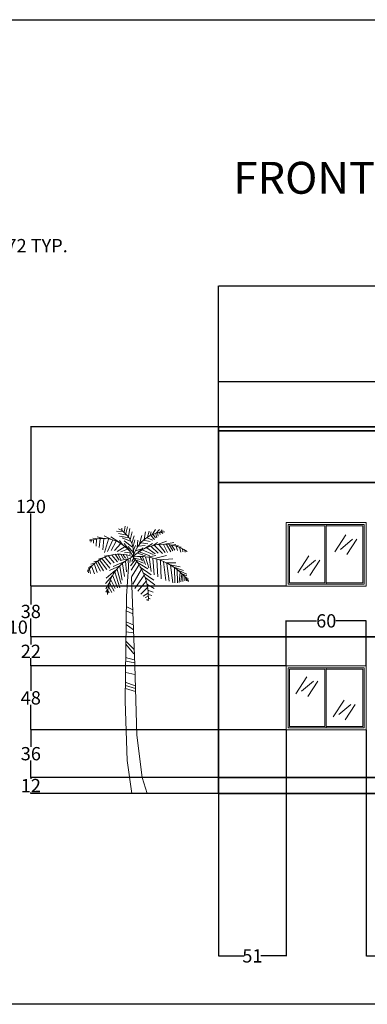
# Model space of a CAD drawing. Units: inches. Extents: x -16 to 1298, y 3 to 744.
# Tile 4 of 5: x 520 to 781, y 3 to 744. Entities that reach past the tile are written whole.
import ezdxf

# ---------------------------------------------------------------- set-up
doc = ezdxf.new("R2010")
doc.units = ezdxf.units.IN
doc.header["$MEASUREMENT"] = 0
for name, color, linetype, lineweight in [('A-ANNO-DIMS', 2, 'Continuous', 18), ('A-ANNO-TITL', 7, 'Continuous', 35), ('A-ELEV', 7, 'Continuous', 35), ('A-GLAZ', 4, 'Continuous', 18), ('A-ROOF', 7, 'Continuous', 35), ('C-TOPO', 7, 'Continuous', 30), ('PLANT', 3, 'Continuous', 13)]:
    doc.layers.add(name, color=color, linetype=linetype, lineweight=lineweight)
doc.styles.get("Standard").update_dxf_attribs({"font": 'arial.ttf'})
doc.dimstyles.get("Standard").update_dxf_attribs({"dimtxt": 10, "dimasz": 0.18, "dimexe": 0.18, "dimexo": 0.0625, "dimgap": 0.09, "dimtad": 0, "dimtih": 1, "dimtoh": 1, "dimdec": 0, "dimzin": 0, "dimdsep": 46, "dimlunit": 3, "dimtxsty": 'Standard', "dimcen": 0.09, "dimadec": 0, "dimazin": 0, "dimtfac": 1, "dimtdec": 0, "dimtofl": 0, "dimtmove": 0, "dimatfit": 3, "dimfxl": 1, "dimtolj": 1, "dimtzin": 0, "dimarcsym": 0})

# ---------------------------------------------------------------- blocks, each defined once
blk = doc.blocks.new('*U11')
for p, q in [((1.5, 1.5), (1.5, 46.5)), ((1.5, 46.5), (30, 46.5)), ((30, 1.5), (30, 46.5)), ((30, 46.5), (58.5, 46.5)), ((58.5, 46.5), (58.5, 1.5)), ((30, 1.5), (1.5, 1.5)), ((58.5, 1.5), (30, 1.5))]:
    blk.add_line(p, q)
blk.add_lwpolyline([(0, 0), (0, 48), (60, 48), (60, 0)], close=True)
for points in [[(29, 45.5), (29, 2.5), (2.5, 2.5), (2.5, 45.5), (29, 45.5)], [(30, 45.5), (57.5, 45.5), (57.5, 2.5), (30, 2.5)]]:
    blk.add_lwpolyline(points)
blk = doc.blocks.new('Tree - palm elevation')
for p, q in [((-5.567, 196.707), (-4.987, 201.167)), ((-4.407, 195.716), (-3.247, 200.672)), ((-20.064, 191.751), (-25.863, 193.238)), ((-15.232, 191.255), (-20.644, 193.981)), ((-9.433, 189.025), (-15.618, 193.238)), ((-6.727, 197.202), (-11.366, 197.45)), ((-3.441, 194.477), (-10.013, 195.716)), ((-1.894, 192.494), (-9.24, 193.733)), ((-7.5, 199.68), (-7.5, 197.946)), ((-2.474, 193.733), (-1.315, 199.433)), ((-1.121, 190.759), (0.232, 196.955)), ((0.038, 188.281), (1.778, 193.981)), ((5.837, 187.786), (7.577, 194.229)), ((9.317, 191.255), (10.283, 196.955)), ((11.829, 192.99), (13.182, 197.45)), ((13.956, 194.229), (14.729, 196.955)), ((14.536, 193.981), (17.242, 191.255)), ((15.116, 194.477), (17.822, 198.689)), ((16.082, 194.972), (17.822, 192.494)), ((18.015, 195.716), (20.914, 198.689)), ((18.015, 195.468), (18.981, 192.494)), ((19.368, 196.459), (19.948, 193.733)), ((20.914, 196.459), (21.301, 194.972)), ((21.301, 196.459), (22.847, 198.441)), ((22.074, 196.707), (23.427, 195.716)), ((23.234, 196.707), (23.62, 197.698)), ((-29.729, 190.759), (-31.469, 191.255)), ((-30.309, 190.512), (-30.695, 189.025)), ((-25.283, 191.751), (-29.342, 192.246)), ((-28.763, 190.759), (-28.763, 188.281)), ((-26.443, 191.503), (-26.636, 186.051)), ((-23.737, 191.751), (-24.51, 185.06)), ((-21.031, 191.998), (-21.804, 183.325)), ((-17.551, 191.503), (-20.451, 181.343)), ((-14.265, 190.759), (-18.131, 182.086)), ((-11.753, 189.768), (-15.425, 182.83)), ((-8.08, 188.034), (-12.912, 182.83)), ((-4.987, 185.803), (-10.979, 182.086)), ((-6.147, 186.299), (-9.24, 190.264)), ((-0.541, 189.52), (-7.307, 192.494)), ((-5.76, 190.016), (0.618, 185.308)), ((-5.76, 188.034), (-1.508, 182.582)), ((-2.668, 185.803), (1.198, 181.343)), ((1.005, 185.803), (2.358, 190.759)), ((1.005, 182.582), (2.938, 186.547)), ((4.098, 185.06), (4.678, 190.512)), ((4.871, 186.051), (10.09, 186.547)), ((6.997, 188.529), (12.216, 187.786)), ((8.544, 190.512), (13.763, 189.52)), ((9.51, 184.317), (15.502, 188.034)), ((11.25, 192.494), (15.889, 190.512)), ((14.536, 185.803), (19.948, 180.847)), ((15.695, 186.299), (19.368, 188.777)), ((17.242, 186.547), (23.041, 180.599)), ((19.368, 187.29), (26.133, 189.768)), ((20.721, 187.042), (25.167, 181.343)), ((23.814, 187.29), (26.907, 181.343)), ((24.78, 187.538), (31.546, 188.777)), ((26.133, 187.29), (29.419, 181.838)), ((28.066, 187.29), (30.966, 182.582)), ((29.806, 186.795), (32.319, 183.078)), ((29.999, 186.795), (33.092, 187.29)), ((32.512, 186.299), (35.218, 186.299)), ((33.479, 186.051), (34.445, 182.83)), ((35.605, 185.556), (37.151, 185.308)), ((35.798, 185.308), (36.958, 181.591)), ((-15.618, 179.36), (-20.644, 178.617)), ((-17.358, 178.617), (-13.299, 173.661)), ((-15.038, 179.36), (-10.786, 174.404)), ((-12.332, 180.104), (-9.433, 175.643)), ((-10.206, 180.104), (-8.08, 175.891)), ((-8.273, 180.104), (-6.147, 176.635)), ((-3.247, 183.821), (-8.08, 181.838)), ((-6.34, 179.608), (-4.6, 177.13)), ((-1.315, 181.591), (-5.374, 181.095)), ((-4.021, 179.36), (-2.861, 177.378)), ((-0.348, 180.352), (-1.894, 180.104)), ((2.938, 182.582), (6.61, 183.821)), ((4.098, 180.847), (8.35, 179.608)), ((4.871, 181.591), (8.544, 184.812)), ((5.644, 181.838), (13.569, 178.865)), ((6.224, 178.121), (8.157, 175.148)), ((7.384, 178.369), (10.476, 179.36)), ((7.77, 183.325), (16.082, 179.856)), ((8.157, 178.121), (10.476, 172.422)), ((10.476, 177.874), (12.796, 169.696)), ((11.25, 184.812), (17.628, 180.352)), ((11.829, 177.874), (18.015, 179.113)), ((13.182, 177.874), (14.729, 166.97)), ((18.015, 177.13), (26.133, 179.113)), ((38.118, 184.317), (38.504, 181.838)), ((39.857, 182.83), (40.244, 181.591)), ((-28.956, 172.174), (-32.435, 170.192)), ((-27.409, 173.413), (-30.695, 172.67)), ((-29.922, 170.687), (-27.989, 165.235)), ((-25.09, 175.148), (-28.376, 174.404)), ((-27.989, 172.422), (-26.056, 166.227)), ((-26.829, 173.661), (-23.544, 167.218)), ((-25.476, 174.652), (-21.224, 167.466)), ((-21.031, 177.626), (-24.897, 176.387)), ((-24.317, 175.891), (-18.711, 168.457)), ((-22.191, 176.635), (-16.391, 169.448)), ((-20.064, 177.626), (-15.812, 172.67)), ((-8.466, 171.678), (-16.585, 167.713)), ((-4.214, 175.148), (-14.072, 170.935)), ((-8.853, 170.935), (-7.113, 160.527)), ((-1.701, 176.882), (-8.66, 175.396)), ((-6.92, 172.917), (-5.374, 163.253)), ((-4.6, 174.9), (-4.021, 166.722)), ((-2.668, 176.387), (-2.376, 170.594)), ((-0.928, 176.882), (-1.508, 173.909)), ((2.551, 175.891), (-0.928, 171.431)), ((3.711, 174.404), (-0.541, 167.961)), ((5.257, 171.926), (-0.155, 163.005)), ((1.585, 177.13), (0.038, 174.652)), ((1.585, 177.13), (6.61, 176.139)), ((2.938, 175.891), (8.737, 173.413)), ((4.291, 173.909), (12.216, 168.953)), ((6.417, 170.439), (14.729, 164.492)), ((15.889, 177.13), (16.855, 164.492)), ((18.981, 175.891), (19.561, 163.005)), ((20.914, 175.891), (30.966, 176.635)), ((21.688, 175.396), (22.074, 161.518)), ((23.814, 174.404), (25.554, 160.279)), ((25.554, 173.661), (33.285, 173.661)), ((26.52, 173.165), (28.066, 159.784)), ((28.839, 172.174), (36.378, 170.687)), ((29.226, 171.926), (30.966, 158.545)), ((30.966, 170.687), (38.891, 167.713)), ((-32.628, 167.961), (-33.208, 167.961)), ((-32.628, 167.713), (-32.435, 165.979)), ((-31.082, 169.944), (-32.435, 169.2)), ((-31.662, 168.705), (-31.082, 165.483)), ((-14.265, 164.244), (-19.678, 158.049)), ((-12.139, 167.961), (-19.098, 162.014)), ((-14.265, 163.749), (-10.786, 154.828)), ((-12.719, 166.722), (-9.046, 154.828)), ((-10.979, 168.457), (-7.887, 157.801)), ((7.384, 168.705), (0.812, 157.553)), ((9.317, 164.244), (2.358, 154.332)), ((8.544, 165.979), (16.662, 160.527)), ((32.126, 169.696), (32.512, 158.545)), ((34.058, 168.705), (34.445, 158.545)), ((35.412, 167.713), (41.404, 164.988)), ((36.378, 166.474), (35.605, 158.792)), ((37.731, 165.235), (36.958, 159.288)), ((37.924, 165.235), (41.404, 163.749)), ((38.504, 164.492), (38.504, 159.536)), ((39.664, 163.253), (42.37, 161.766)), ((-16.005, 160.031), (-19.484, 154.084)), ((-17.358, 155.819), (-14.845, 151.358)), ((-16.585, 158.545), (-13.106, 152.35)), ((-15.618, 160.775), (-12.332, 154.332)), ((10.863, 159.784), (4.484, 152.35)), ((10.09, 162.51), (17.435, 157.058)), ((11.443, 157.553), (16.855, 154.332)), ((39.857, 162.757), (39.857, 160.031)), ((40.824, 161.766), (41.21, 160.031)), ((41.21, 161.518), (42.757, 160.279)), ((-18.131, 153.589), (-19.484, 151.606)), ((-17.938, 152.597), (-16.972, 151.111)), ((11.829, 155.075), (6.804, 150.119)), ((12.603, 151.111), (8.544, 148.385)), ((12.216, 153.093), (16.082, 151.606)), ((12.603, 149.872), (15.116, 149.128)), ((12.216, 148.137), (10.09, 147.393)), ((12.409, 145.659), (11.056, 145.659)), ((12.409, 146.898), (13.763, 146.402)), ((-4.081, 140.645), (0.753, 138.261)), ((-4.081, 137.547), (0.753, 135.163)), ((-4.081, 129.205), (1.124, 126.821)), ((-4.081, 127.298), (1.31, 123.246)), ((-4.081, 121.578), (1.31, 120.863)), ((-4.453, 112.283), (1.682, 105.133)), ((-4.267, 114.428), (1.682, 108.708)), ((-4.639, 102.273), (1.868, 100.604)), ((-4.453, 99.651), (2.24, 98.459)), ((-4.453, 91.071), (2.426, 89.641)), ((-4.825, 83.921), (2.612, 81.061)), ((-4.639, 81.299), (2.797, 78.916)), ((-4.639, 78.916), (2.797, 76.771))]:
    blk.add_line(p, q)
for points in [[(-2.363, 170.553), (-3.88, 148.505), (-4.988, 69.634), (-3.325, 24.869), (0, 0)], [(-0.116, 162.848), (0.554, 143.532), (2.217, 96.635), (3.88, 44.054), (7.76, 12.079), (11.64, 0)]]:
    blk.add_lwpolyline(points)
for centre, radius, start, end in [((-18.427, 181.448), 19.715, 350.285, 64.11229), ((25.595, 171.567), 25.395, 91.40319, 163.882), ((-21.738, 166.094), 25.899, 27.67115, 112.5305), ((23.687, 155.341), 32.188, 56.19272, 134.3213), ((-9.259, 151.732), 28.386, 68.38311, 147.5322), ((14.394, 148.393), 32.752, 113.7592, 177.4133), ((5.828, 132.718), 45.639, 35.98777, 95.82273), ((-32.8, 147.923), 45.309, 356.1943, 41.37848)]:
    blk.add_arc(centre, radius, start, end)
blk = doc.blocks.new('GLASS-REFLECTION-LARGE')
for p, q in [((8.29, 14.77), (0, 2.16)), ((13.34, 11.53), (4.33, 3.96)), ((16.59, 11.53), (9.01, 0))]:
    blk.add_line(p, q)
blk = doc.blocks.new('*D26')
at = {"layer": 'A-ANNO-DIMS', "color": 0, "lineweight": -2, "transparency": 16777216}
for p, q in [((373.61, 584.93), (373.61, 574.01)), ((445.61, 584.93), (445.61, 574.01)), ((373.79, 574.19), (445.43, 574.19)), ((445.61, 574.19), (445.79, 574.19))]:
    blk.add_line(p, q, dxfattribs=at)
at = {"layer": 'A-ANNO-DIMS', "color": 0, "transparency": 16777216}
for points in [[(373.79, 574.22), (373.79, 574.16), (373.61, 574.19)], [(445.43, 574.22), (445.43, 574.16), (445.61, 574.19)]]:
    blk.add_solid(points, dxfattribs=at)
at = {"layer": 'Defpoints', "color": 0, "transparency": 16777216}
for p in [(373.61, 584.99), (445.61, 584.99), (445.61, 574.19)]:
    blk.add_point(p, dxfattribs=at)
at = {"layer": 'A-ANNO-DIMS', "color": 0, "transparency": 16777216, "insert": (503.01, 574.19), "char_height": 10, "attachment_point": 5}
blk.add_mtext('\\A1;WINDOW 72 TYP.', dxfattribs=at)
blk = doc.blocks.new('*D44')
at = {"layer": 'A-ANNO-DIMS', "color": 0, "lineweight": -2, "transparency": 16777216}
for p, q in [((478.74, 286.99), (511.91, 286.99)), ((511.73, 286.99), (511.73, 287.17)), ((511.73, 287.17), (511.91, 287.17)), ((511.73, 277.17), (511.73, 286.81)), ((478.74, 276.99), (511.91, 276.99))]:
    blk.add_line(p, q, dxfattribs=at)
at = {"layer": 'A-ANNO-DIMS', "color": 0, "transparency": 16777216}
for points in [[(511.7, 286.81), (511.76, 286.81), (511.73, 286.99)], [(511.7, 277.17), (511.76, 277.17), (511.73, 276.99)]]:
    blk.add_solid(points, dxfattribs=at)
at = {"layer": 'Defpoints', "color": 0, "transparency": 16777216}
for p in [(478.68, 286.99), (511.73, 286.99), (478.68, 276.99)]:
    blk.add_point(p, dxfattribs=at)
at = {"layer": 'A-ANNO-DIMS', "color": 0, "transparency": 16777216, "insert": (518.67, 287.17), "char_height": 10, "attachment_point": 5}
blk.add_mtext('\\A1;10', dxfattribs=at)
blk = doc.blocks.new('*D63')
at = {"layer": 'A-ANNO-DIMS', "color": 0, "lineweight": -2, "transparency": 16777216}
for p, q in [((669.53, 438.05), (669.53, 544.07)), ((669.71, 543.89), (850.42, 543.89)), ((1053.35, 543.89), (872.64, 543.89)), ((1053.53, 510.05), (1053.53, 544.07))]:
    blk.add_line(p, q, dxfattribs=at)
at = {"layer": 'A-ANNO-DIMS', "color": 0, "transparency": 16777216}
for points in [[(669.71, 543.92), (669.71, 543.86), (669.53, 543.89)], [(1053.35, 543.92), (1053.35, 543.86), (1053.53, 543.89)]]:
    blk.add_solid(points, dxfattribs=at)
at = {"layer": 'Defpoints', "color": 0, "transparency": 16777216}
for p in [(1053.53, 543.89), (1053.53, 509.99), (669.53, 437.99)]:
    blk.add_point(p, dxfattribs=at)
at = {"layer": 'A-ANNO-DIMS', "color": 0, "transparency": 16777216, "insert": (861.53, 543.89), "char_height": 10, "attachment_point": 5}
blk.add_mtext('\\A1;384', dxfattribs=at)
blk = doc.blocks.new('*D65')
at = {"layer": 'A-ANNO-DIMS', "color": 0, "lineweight": -2, "transparency": 16777216}
for p, q in [((669.47, 173.99), (528.28, 173.99)), ((528.46, 173.81), (528.46, 173.1)), ((669.47, 161.99), (528.28, 161.99)), ((528.46, 162.17), (528.46, 162.88))]:
    blk.add_line(p, q, dxfattribs=at)
at = {"layer": 'A-ANNO-DIMS', "color": 0, "transparency": 16777216}
for points in [[(528.43, 173.81), (528.49, 173.81), (528.46, 173.99)], [(528.43, 162.17), (528.49, 162.17), (528.46, 161.99)]]:
    blk.add_solid(points, dxfattribs=at)
at = {"layer": 'Defpoints', "color": 0, "transparency": 16777216}
for p in [(528.46, 173.99), (669.53, 173.99), (669.53, 161.99)]:
    blk.add_point(p, dxfattribs=at)
at = {"layer": 'A-ANNO-DIMS', "color": 0, "transparency": 16777216, "insert": (528.46, 167.99), "char_height": 10, "attachment_point": 5}
blk.add_mtext('\\A1;12', dxfattribs=at)
blk = doc.blocks.new('*D66')
at = {"layer": 'A-ANNO-DIMS', "color": 0, "lineweight": -2, "transparency": 16777216}
for p, q in [((720.47, 209.99), (528.28, 209.99)), ((528.46, 209.81), (528.46, 197.19)), ((528.46, 174.17), (528.46, 186.79)), ((669.47, 173.99), (528.28, 173.99))]:
    blk.add_line(p, q, dxfattribs=at)
at = {"layer": 'A-ANNO-DIMS', "color": 0, "transparency": 16777216}
for points in [[(528.43, 209.81), (528.49, 209.81), (528.46, 209.99)], [(528.43, 174.17), (528.49, 174.17), (528.46, 173.99)]]:
    blk.add_solid(points, dxfattribs=at)
at = {"layer": 'Defpoints', "color": 0, "transparency": 16777216}
for p in [(528.46, 209.99), (720.53, 209.99), (669.53, 173.99)]:
    blk.add_point(p, dxfattribs=at)
at = {"layer": 'A-ANNO-DIMS', "color": 0, "transparency": 16777216, "insert": (528.46, 191.99), "char_height": 10, "attachment_point": 5}
blk.add_mtext('\\A1;36', dxfattribs=at)
blk = doc.blocks.new('*D67')
at = {"layer": 'A-ANNO-DIMS', "color": 0, "lineweight": -2, "transparency": 16777216}
for p, q in [((720.47, 257.99), (528.28, 257.99)), ((528.46, 257.81), (528.46, 239.18)), ((528.46, 210.17), (528.46, 228.79)), ((720.47, 209.99), (528.28, 209.99))]:
    blk.add_line(p, q, dxfattribs=at)
at = {"layer": 'A-ANNO-DIMS', "color": 0, "transparency": 16777216}
for points in [[(528.43, 257.81), (528.49, 257.81), (528.46, 257.99)], [(528.43, 210.17), (528.49, 210.17), (528.46, 209.99)]]:
    blk.add_solid(points, dxfattribs=at)
at = {"layer": 'Defpoints', "color": 0, "transparency": 16777216}
for p in [(528.46, 257.99), (720.53, 257.99), (720.53, 209.99)]:
    blk.add_point(p, dxfattribs=at)
at = {"layer": 'A-ANNO-DIMS', "color": 0, "transparency": 16777216, "insert": (528.46, 233.99), "char_height": 10, "attachment_point": 5}
blk.add_mtext('\\A1;48', dxfattribs=at)
blk = doc.blocks.new('*D68')
at = {"layer": 'A-ANNO-DIMS', "color": 0, "lineweight": -2, "transparency": 16777216}
for p, q in [((669.47, 279.99), (528.28, 279.99)), ((528.46, 279.81), (528.46, 274.1)), ((528.46, 258.17), (528.46, 263.88)), ((720.47, 257.99), (528.28, 257.99))]:
    blk.add_line(p, q, dxfattribs=at)
at = {"layer": 'A-ANNO-DIMS', "color": 0, "transparency": 16777216}
for points in [[(528.43, 279.81), (528.49, 279.81), (528.46, 279.99)], [(528.43, 258.17), (528.49, 258.17), (528.46, 257.99)]]:
    blk.add_solid(points, dxfattribs=at)
at = {"layer": 'Defpoints', "color": 0, "transparency": 16777216}
for p in [(528.46, 279.99), (669.53, 279.99), (720.53, 257.99)]:
    blk.add_point(p, dxfattribs=at)
at = {"layer": 'A-ANNO-DIMS', "color": 0, "transparency": 16777216, "insert": (528.46, 268.99), "char_height": 10, "attachment_point": 5}
blk.add_mtext('\\A1;22', dxfattribs=at)
blk = doc.blocks.new('*D69')
at = {"layer": 'A-ANNO-DIMS', "color": 0, "lineweight": -2, "transparency": 16777216}
for p, q in [((720.47, 317.99), (528.28, 317.99)), ((528.46, 317.81), (528.46, 304.19)), ((528.46, 280.17), (528.46, 293.79)), ((669.47, 279.99), (528.28, 279.99))]:
    blk.add_line(p, q, dxfattribs=at)
at = {"layer": 'A-ANNO-DIMS', "color": 0, "transparency": 16777216}
for points in [[(528.43, 317.81), (528.49, 317.81), (528.46, 317.99)], [(528.43, 280.17), (528.49, 280.17), (528.46, 279.99)]]:
    blk.add_solid(points, dxfattribs=at)
at = {"layer": 'Defpoints', "color": 0, "transparency": 16777216}
for p in [(528.46, 317.99), (720.53, 317.99), (669.53, 279.99)]:
    blk.add_point(p, dxfattribs=at)
at = {"layer": 'A-ANNO-DIMS', "color": 0, "transparency": 16777216, "insert": (528.46, 298.99), "char_height": 10, "attachment_point": 5}
blk.add_mtext('\\A1;38', dxfattribs=at)
blk = doc.blocks.new('*D70')
at = {"layer": 'A-ANNO-DIMS', "color": 0, "lineweight": -2, "transparency": 16777216}
for p, q in [((669.47, 437.99), (528.28, 437.99)), ((528.46, 437.81), (528.46, 383.18)), ((528.46, 318.17), (528.46, 372.79)), ((720.47, 317.99), (528.28, 317.99))]:
    blk.add_line(p, q, dxfattribs=at)
at = {"layer": 'A-ANNO-DIMS', "color": 0, "transparency": 16777216}
for points in [[(528.43, 437.81), (528.49, 437.81), (528.46, 437.99)], [(528.43, 318.17), (528.49, 318.17), (528.46, 317.99)]]:
    blk.add_solid(points, dxfattribs=at)
at = {"layer": 'Defpoints', "color": 0, "transparency": 16777216}
for p in [(528.46, 437.99), (669.53, 437.99), (720.53, 317.99)]:
    blk.add_point(p, dxfattribs=at)
at = {"layer": 'A-ANNO-DIMS', "color": 0, "transparency": 16777216, "insert": (528.46, 377.99), "char_height": 10, "attachment_point": 5}
blk.add_mtext('\\A1;120', dxfattribs=at)
blk = doc.blocks.new('*D72')
at = {"layer": 'A-ANNO-DIMS', "color": 0, "lineweight": -2, "transparency": 16777216}
for p, q in [((720.53, 209.93), (720.53, 39.71)), ((669.53, 173.93), (669.53, 39.71)), ((669.71, 39.89), (688.74, 39.89)), ((720.35, 39.89), (701.32, 39.89))]:
    blk.add_line(p, q, dxfattribs=at)
at = {"layer": 'A-ANNO-DIMS', "color": 0, "transparency": 16777216}
for points in [[(669.71, 39.92), (669.71, 39.86), (669.53, 39.89)], [(720.35, 39.92), (720.35, 39.86), (720.53, 39.89)]]:
    blk.add_solid(points, dxfattribs=at)
at = {"layer": 'Defpoints', "color": 0, "transparency": 16777216}
for p in [(720.53, 209.99), (669.53, 173.99), (720.53, 39.89)]:
    blk.add_point(p, dxfattribs=at)
at = {"layer": 'A-ANNO-DIMS', "color": 0, "transparency": 16777216, "insert": (695.03, 39.89), "char_height": 10, "attachment_point": 5}
blk.add_mtext('\\A1;51', dxfattribs=at)
blk = doc.blocks.new('*D73')
at = {"layer": 'A-ANNO-DIMS', "color": 0, "lineweight": -2, "transparency": 16777216}
for p, q in [((720.53, 258.05), (720.53, 292.07)), ((720.71, 291.89), (743.27, 291.89)), ((780.35, 291.89), (757.79, 291.89)), ((780.53, 258.05), (780.53, 292.07))]:
    blk.add_line(p, q, dxfattribs=at)
at = {"layer": 'A-ANNO-DIMS', "color": 0, "transparency": 16777216}
for points in [[(720.71, 291.92), (720.71, 291.86), (720.53, 291.89)], [(780.35, 291.92), (780.35, 291.86), (780.53, 291.89)]]:
    blk.add_solid(points, dxfattribs=at)
at = {"layer": 'Defpoints', "color": 0, "transparency": 16777216}
for p in [(780.53, 291.89), (720.53, 257.99), (780.53, 257.99)]:
    blk.add_point(p, dxfattribs=at)
at = {"layer": 'A-ANNO-DIMS', "color": 0, "transparency": 16777216, "insert": (750.53, 291.89), "char_height": 10, "attachment_point": 5}
blk.add_mtext('\\A1;60', dxfattribs=at)
blk = doc.blocks.new('*D74')
at = {"layer": 'A-ANNO-DIMS', "color": 0, "lineweight": -2, "transparency": 16777216}
for p, q in [((780.53, 209.93), (780.53, 39.71)), ((884.37, 173.94), (884.37, 39.71)), ((780.71, 39.89), (812.09, 39.89)), ((884.19, 39.89), (852.8, 39.89))]:
    blk.add_line(p, q, dxfattribs=at)
at = {"layer": 'A-ANNO-DIMS', "color": 0, "transparency": 16777216}
for points in [[(780.71, 39.92), (780.71, 39.86), (780.53, 39.89)], [(884.19, 39.92), (884.19, 39.86), (884.37, 39.89)]]:
    blk.add_solid(points, dxfattribs=at)
at = {"layer": 'Defpoints', "color": 0, "transparency": 16777216}
for p in [(780.53, 209.99), (884.37, 174), (884.37, 39.89)]:
    blk.add_point(p, dxfattribs=at)
at = {"layer": 'A-ANNO-DIMS', "color": 0, "transparency": 16777216, "insert": (832.45, 39.89), "char_height": 10, "attachment_point": 5}
blk.add_mtext('\\A1;103.84', dxfattribs=at)
blk = doc.blocks.new('*D81')
at = {"layer": 'A-ANNO-DIMS', "color": 0, "lineweight": -2, "transparency": 16777216}
for p, q in [((669.53, 438.05), (669.53, 472.07)), ((669.71, 471.89), (808.41, 471.89)), ((969.35, 471.89), (830.65, 471.89)), ((969.53, 438.05), (969.53, 472.07))]:
    blk.add_line(p, q, dxfattribs=at)
at = {"layer": 'A-ANNO-DIMS', "color": 0, "transparency": 16777216}
for points in [[(669.71, 471.92), (669.71, 471.86), (669.53, 471.89)], [(969.35, 471.92), (969.35, 471.86), (969.53, 471.89)]]:
    blk.add_solid(points, dxfattribs=at)
at = {"layer": 'Defpoints', "color": 0, "transparency": 16777216}
for p in [(969.53, 471.89), (669.53, 437.99), (969.53, 437.99)]:
    blk.add_point(p, dxfattribs=at)
at = {"layer": 'A-ANNO-DIMS', "color": 0, "transparency": 16777216, "insert": (819.53, 471.89), "char_height": 10, "attachment_point": 5}
blk.add_mtext('\\A1;300', dxfattribs=at)

msp = doc.modelspace()

# ---------------------------------------------------------------- linework, layer by layer
at = {"layer": 'A-ELEV'}
for p, q in [((669.5287, 161.9884), (669.5287, 437.9884)), ((828.5287, 395.9884), (669.5287, 395.9884)), ((827.5287, 279.9884), (669.5287, 279.9884)), ((1041.5287, 173.9884), (669.5287, 173.9884)), ((823.5287, 161.9884), (669.5287, 161.9884))]:
    msp.add_line(p, q, dxfattribs=at)
at = {"layer": 'A-ROOF'}
for p, q in [((993.5287, 437.9884), (669.5287, 437.9884)), ((993.5287, 434.9884), (669.5287, 434.9884))]:
    msp.add_line(p, q, dxfattribs=at)
at = {"layer": 'C-TOPO'}
msp.add_line((669.5287, 161.9884), (562.3611, 161.9884), dxfattribs=at)
at = {"layer": 'Defpoints'}
msp.add_lwpolyline([(8.9336, 744.17), (1298.346, 744.17), (1298.346, 3.4476), (8.9336, 3.4476)], close=True, dxfattribs=at)

# ---------------------------------------------------------------- block references
at = {"layer": 'A-GLAZ'}
for name, p in [('*U11', (720.5287, 317.9884)), ('GLASS-REFLECTION-LARGE', (756.9184, 341.7425)), ('GLASS-REFLECTION-LARGE', (729.2063, 325.9811)), ('*U11', (720.5287, 209.9884)), ('GLASS-REFLECTION-LARGE', (727.6977, 234.9468)), ('GLASS-REFLECTION-LARGE', (755.7111, 217.4985))]:
    msp.add_blockref(name, p, dxfattribs=at)
at = {"layer": 'PLANT'}
msp.add_blockref('Tree - palm elevation', (604.3049, 161.9884), dxfattribs=at)

# ---------------------------------------------------------------- texts
at = {"layer": 'A-ANNO-TITL', "insert": (680.7425, 637.2274), "char_height": 24, "attachment_point": 1}
msp.add_mtext_dynamic_manual_height_columns('{\\fTimes New Roman|b0|i0|c0|p18;FRONT ELEVATION}', width=347.060427, gutter_width=1, heights=[0], dxfattribs=at)

# ---------------------------------------------------------------- dimensions: what is measured, and where the dimension line sits
at = {"layer": 'A-ANNO-DIMS'}
dim = msp.add_linear_dim(base=(445.6051, 574.1884), p1=(373.6051, 584.9884), p2=(445.6051, 584.9884), text='WINDOW <> TYP.', dimstyle='Standard', override={"dimdec": 0, "dimlfac": 1, "dimrnd": 0, "dimzin": 0, "dimdsep": 46, "dimlunit": 2}, dxfattribs=at)
dim.commit()
dim.dimension.update_dxf_attribs({"geometry": '*D26', "text_midpoint": (503.0068, 574.1884)})
for base, p1, p2, override, picture, middle in [((1053.5287, 543.8884), (669.5287, 437.9884), (1053.5287, 509.9884), {"dimdec": 0, "dimlfac": 1, "dimrnd": 0, "dimzin": 0, "dimdsep": 46, "dimlunit": 2}, '*D63', (861.5287, 543.8884)), ((969.5287, 471.8884), (669.5287, 437.9884), (969.5287, 437.9884), {"dimdec": 0, "dimlfac": 1, "dimrnd": 0, "dimzin": 0, "dimdsep": 46, "dimlunit": 2}, '*D81', (819.5287, 471.8884)), ((780.5287, 291.8884), (720.5287, 257.9884), (780.5287, 257.9884), {"dimdec": 0, "dimlfac": 1, "dimrnd": 0, "dimzin": 0, "dimdsep": 46, "dimlunit": 2}, '*D73', (750.5287, 291.8884)), ((720.5287, 39.894), (669.5287, 173.9884), (720.5287, 209.9884), {"dimdec": 0, "dimlfac": 1, "dimrnd": 0, "dimzin": 0, "dimdsep": 46, "dimlunit": 2}, '*D72', (695.0287, 39.894)), ((884.3677, 39.894), (780.5287, 209.9884), (884.3677, 174.0011), {"dimdec": 2, "dimlfac": 1, "dimrnd": 0, "dimzin": 0, "dimdsep": 46, "dimlunit": 2}, '*D74', (832.4482, 39.894))]:
    dim = msp.add_linear_dim(base=base, p1=p1, p2=p2, dimstyle='Standard', override=override, dxfattribs=at)
    dim.commit()
    dim.dimension.update_dxf_attribs({"geometry": picture, "text_midpoint": middle})
for base, p1, p2, picture, middle in [((528.4611, 437.9884), (720.5287, 317.9884), (669.5287, 437.9884), '*D70', (528.4611, 377.9884)), ((528.4611, 317.9884), (669.5287, 279.9884), (720.5287, 317.9884), '*D69', (528.4611, 298.9884)), ((511.7268, 286.9884), (478.6768, 276.9884), (478.6768, 286.9884), '*D44', (518.6714, 287.1684)), ((528.4611, 279.9884), (720.5287, 257.9884), (669.5287, 279.9884), '*D68', (528.4611, 268.9884)), ((528.4611, 257.9884), (720.5287, 209.9884), (720.5287, 257.9884), '*D67', (528.4611, 233.9884)), ((528.4611, 209.9884), (669.5287, 173.9884), (720.5287, 209.9884), '*D66', (528.4611, 191.9884)), ((528.4611, 173.9884), (669.5287, 161.9884), (669.5287, 173.9884), '*D65', (528.4611, 167.9884))]:
    dim = msp.add_linear_dim(base=base, p1=p1, p2=p2, angle=90, dimstyle='Standard', override={"dimdec": 0, "dimlfac": 1, "dimrnd": 0, "dimzin": 0, "dimdsep": 46, "dimlunit": 2}, dxfattribs=at)
    dim.commit()
    dim.dimension.update_dxf_attribs({"geometry": picture, "text_midpoint": middle})

doc.saveas('drawing.dxf')
